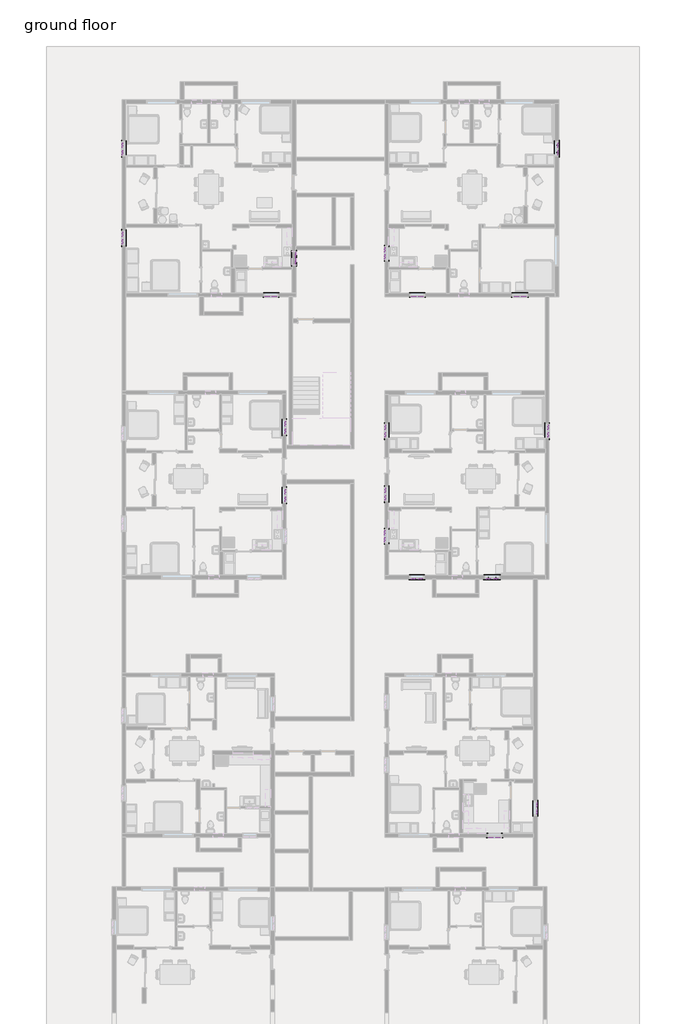
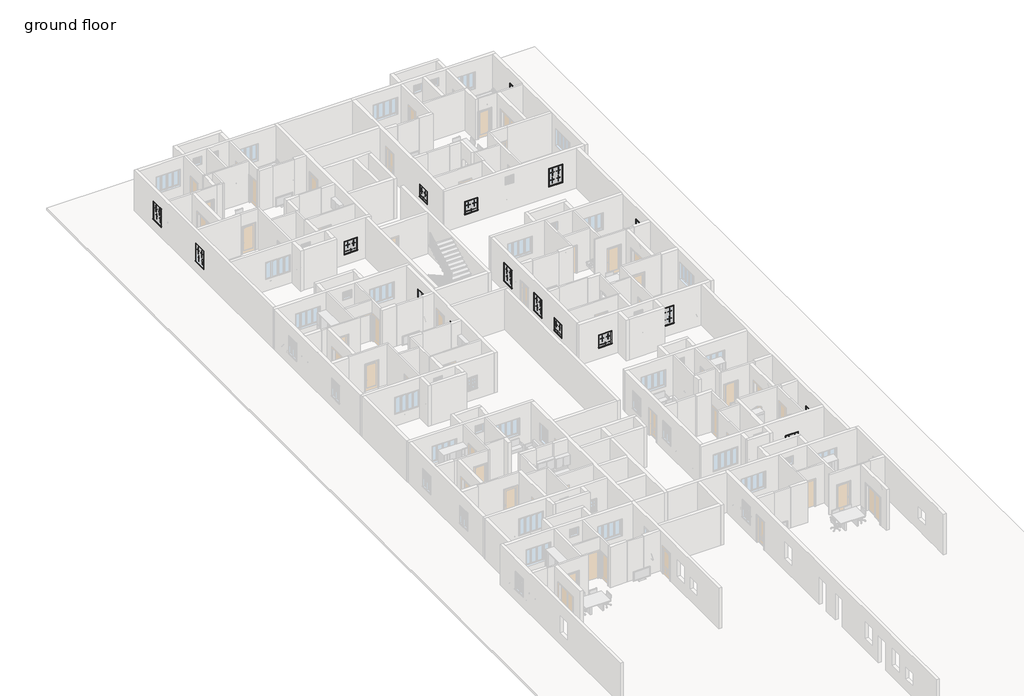
# One storey, part 16 of 16: 100 proxies.
"""IFC4 building model written with IfcOpenShell, lengths in millimetres."""

from ifc_helpers import new_model, si_unit, origin, place, context, project, spatial, transform, mapped, element, save
from components import muntin_pattern_2x2_muntin_pattern_2x2_cd1db81d, muntin_pattern_2x2_muntin_pattern_2x2_7c797e2d, muntin_pattern_2x2_muntin_pattern_2x2_78ce0566, muntin_pattern_2x2_muntin_pattern_2x2_27bf4e5b, muntin_pattern_2x2_muntin_pattern_2x2_8320156c, trim_window_exterior_flat_with_sill_fadbc092, trim_window_exterior_flat_with_sill_41619996, trim_window_interior_flat_picture_frame_db6fc9b7, trim_window_interior_flat_picture_frame_51c85655

model = new_model("IFC4")

# Units and contexts
model_context = context("Model", 3, world=origin())
ifc_project = project(units=[si_unit("LENGTHUNIT", "METRE", prefix="MILLI")], contexts=[model_context])

# Site, building, storey
site = spatial("IfcSite", under=ifc_project)
building = spatial("IfcBuilding", under=site)
storey = spatial("IfcBuildingStorey", under=building, Name="ground floor", Elevation=609.6)

# Proxies
placement = place(None, origin())
muntin_pattern_2x2_muntin_pattern_2x2_shape = muntin_pattern_2x2_muntin_pattern_2x2_cd1db81d(model_context)
element("IfcBuildingElementProxy", 1, Name="Muntin Pattern_2x2 : Muntin Pattern_2x2", ObjectType="Muntin Pattern_2x2 : Muntin Pattern_2x2", at=placement, inside=storey, context=model_context, shape_type="MappedRepresentation", body=[
    mapped(muntin_pattern_2x2_muntin_pattern_2x2_shape, transform((43176.551243, 42287.5965635, 2206.625), x_axis=(0.0, 1.0, 0.0), y_axis=(-1.0, 0.0, 0.0), z_axis=(0.0, 0.0, 1.0))),
])
element("IfcBuildingElementProxy", 2, Name="Muntin Pattern_2x2 : Muntin Pattern_2x2", ObjectType="Muntin Pattern_2x2 : Muntin Pattern_2x2", at=placement, inside=storey, context=model_context, shape_type="MappedRepresentation", body=[
    mapped(muntin_pattern_2x2_muntin_pattern_2x2_shape, transform((43221.001243, 42287.5965635, 1600.2), x_axis=(0.0, 1.0, 0.0), y_axis=(-1.0, 0.0, 0.0), z_axis=(0.0, 0.0, 1.0))),
])
element("IfcBuildingElementProxy", 3, Name="Muntin Pattern_2x2 : Muntin Pattern_2x2", ObjectType="Muntin Pattern_2x2 : Muntin Pattern_2x2", at=placement, inside=storey, context=model_context, shape_type="MappedRepresentation", body=[
    mapped(muntin_pattern_2x2_muntin_pattern_2x2_shape, transform((43176.551243, 47785.5373351, 2206.625), x_axis=(0.0, 1.0, 0.0), y_axis=(-1.0, 0.0, 0.0), z_axis=(0.0, 0.0, 1.0))),
])
element("IfcBuildingElementProxy", 4, Name="Muntin Pattern_2x2 : Muntin Pattern_2x2", ObjectType="Muntin Pattern_2x2 : Muntin Pattern_2x2", at=placement, inside=storey, context=model_context, shape_type="MappedRepresentation", body=[
    mapped(muntin_pattern_2x2_muntin_pattern_2x2_shape, transform((43221.001243, 47785.5373351, 1600.2), x_axis=(0.0, 1.0, 0.0), y_axis=(-1.0, 0.0, 0.0), z_axis=(0.0, 0.0, 1.0))),
])
element("IfcBuildingElementProxy", 5, Name="Muntin Pattern_2x2 : Muntin Pattern_2x2", ObjectType="Muntin Pattern_2x2 : Muntin Pattern_2x2", at=placement, inside=storey, context=model_context, shape_type="MappedRepresentation", body=[
    mapped(muntin_pattern_2x2_muntin_pattern_2x2_shape, transform((67459.9250319, 38468.5059867, 2206.625), x_axis=(-1.0, 0.0, 0.0), y_axis=(0.0, -1.0, 0.0), z_axis=(0.0, 0.0, 1.0))),
])
element("IfcBuildingElementProxy", 6, Name="Muntin Pattern_2x2 : Muntin Pattern_2x2", ObjectType="Muntin Pattern_2x2 : Muntin Pattern_2x2", at=placement, inside=storey, context=model_context, shape_type="MappedRepresentation", body=[
    mapped(muntin_pattern_2x2_muntin_pattern_2x2_shape, transform((67459.9250319, 38512.9559867, 1600.2), x_axis=(-1.0, 0.0, 0.0), y_axis=(0.0, -1.0, 0.0), z_axis=(0.0, 0.0, 1.0))),
])
element("IfcBuildingElementProxy", 7, Name="Muntin Pattern_2x2 : Muntin Pattern_2x2", ObjectType="Muntin Pattern_2x2 : Muntin Pattern_2x2", at=placement, inside=storey, context=model_context, shape_type="MappedRepresentation", body=[
    mapped(muntin_pattern_2x2_muntin_pattern_2x2_shape, transform((70050.1113207, 47329.9248351, 2206.625), x_axis=(0.0, -1.0, 0.0), y_axis=(1.0, 0.0, 0.0), z_axis=(0.0, 0.0, 1.0))),
])
element("IfcBuildingElementProxy", 8, Name="Muntin Pattern_2x2 : Muntin Pattern_2x2", ObjectType="Muntin Pattern_2x2 : Muntin Pattern_2x2", at=placement, inside=storey, context=model_context, shape_type="MappedRepresentation", body=[
    mapped(muntin_pattern_2x2_muntin_pattern_2x2_shape, transform((70005.6613207, 47329.9248351, 1600.2), x_axis=(0.0, -1.0, 0.0), y_axis=(1.0, 0.0, 0.0), z_axis=(0.0, 0.0, 1.0))),
])
element("IfcBuildingElementProxy", 9, Name="Muntin Pattern_2x2 : Muntin Pattern_2x2", ObjectType="Muntin Pattern_2x2 : Muntin Pattern_2x2", at=placement, inside=storey, context=model_context, shape_type="MappedRepresentation", body=[
    mapped(muntin_pattern_2x2_muntin_pattern_2x2_shape, transform((69443.5062819, 29924.6588152, 2206.625), x_axis=(0.0, -1.0, 0.0), y_axis=(1.0, 0.0, 0.0), z_axis=(0.0, 0.0, 1.0))),
])
element("IfcBuildingElementProxy", 10, Name="Muntin Pattern_2x2 : Muntin Pattern_2x2", ObjectType="Muntin Pattern_2x2 : Muntin Pattern_2x2", at=placement, inside=storey, context=model_context, shape_type="MappedRepresentation", body=[
    mapped(muntin_pattern_2x2_muntin_pattern_2x2_shape, transform((69399.0562819, 29924.6588152, 1600.2), x_axis=(0.0, -1.0, 0.0), y_axis=(1.0, 0.0, 0.0), z_axis=(0.0, 0.0, 1.0))),
])
element("IfcBuildingElementProxy", 11, Name="Muntin Pattern_2x2 : Muntin Pattern_2x2", ObjectType="Muntin Pattern_2x2 : Muntin Pattern_2x2", at=placement, inside=storey, context=model_context, shape_type="MappedRepresentation", body=[
    mapped(muntin_pattern_2x2_muntin_pattern_2x2_shape, transform((59391.4562819, 26494.0713152, 2206.625), x_axis=(0.0, 1.0, 0.0), y_axis=(-1.0, 0.0, 0.0), z_axis=(0.0, 0.0, 1.0))),
])
element("IfcBuildingElementProxy", 12, Name="Muntin Pattern_2x2 : Muntin Pattern_2x2", ObjectType="Muntin Pattern_2x2 : Muntin Pattern_2x2", at=placement, inside=storey, context=model_context, shape_type="MappedRepresentation", body=[
    mapped(muntin_pattern_2x2_muntin_pattern_2x2_shape, transform((59435.9062819, 26494.0713152, 1600.2), x_axis=(0.0, 1.0, 0.0), y_axis=(-1.0, 0.0, 0.0), z_axis=(0.0, 0.0, 1.0))),
])
element("IfcBuildingElementProxy", 13, Name="Muntin Pattern_2x2 : Muntin Pattern_2x2", ObjectType="Muntin Pattern_2x2 : Muntin Pattern_2x2", at=placement, inside=storey, context=model_context, shape_type="MappedRepresentation", body=[
    mapped(muntin_pattern_2x2_muntin_pattern_2x2_shape, transform((65744.5920559, 21056.0900652, 2206.625), x_axis=(-1.0, 0.0, 0.0), y_axis=(0.0, -1.0, 0.0), z_axis=(0.0, 0.0, 1.0))),
])
element("IfcBuildingElementProxy", 14, Name="Muntin Pattern_2x2 : Muntin Pattern_2x2", ObjectType="Muntin Pattern_2x2 : Muntin Pattern_2x2", at=placement, inside=storey, context=model_context, shape_type="MappedRepresentation", body=[
    mapped(muntin_pattern_2x2_muntin_pattern_2x2_shape, transform((65744.5920559, 21100.5400652, 1600.2), x_axis=(-1.0, 0.0, 0.0), y_axis=(0.0, -1.0, 0.0), z_axis=(0.0, 0.0, 1.0))),
])
element("IfcBuildingElementProxy", 15, Name="Muntin Pattern_2x2 : Muntin Pattern_2x2", ObjectType="Muntin Pattern_2x2 : Muntin Pattern_2x2", at=placement, inside=storey, context=model_context, shape_type="MappedRepresentation", body=[
    mapped(muntin_pattern_2x2_muntin_pattern_2x2_shape, transform((53228.601243, 25959.8281764, 2206.625), x_axis=(0.0, -1.0, 0.0), y_axis=(1.0, 0.0, 0.0), z_axis=(0.0, 0.0, 1.0))),
])
element("IfcBuildingElementProxy", 16, Name="Muntin Pattern_2x2 : Muntin Pattern_2x2", ObjectType="Muntin Pattern_2x2 : Muntin Pattern_2x2", at=placement, inside=storey, context=model_context, shape_type="MappedRepresentation", body=[
    mapped(muntin_pattern_2x2_muntin_pattern_2x2_shape, transform((53184.151243, 25959.8281764, 1600.2), x_axis=(0.0, -1.0, 0.0), y_axis=(1.0, 0.0, 0.0), z_axis=(0.0, 0.0, 1.0))),
])
element("IfcBuildingElementProxy", 17, Name="Muntin Pattern_2x2 : Muntin Pattern_2x2", ObjectType="Muntin Pattern_2x2 : Muntin Pattern_2x2", at=placement, inside=storey, context=model_context, shape_type="MappedRepresentation", body=[
    mapped(muntin_pattern_2x2_muntin_pattern_2x2_shape, transform((53228.601243, 30153.2588152, 2206.625), x_axis=(0.0, -1.0, 0.0), y_axis=(1.0, 0.0, 0.0), z_axis=(0.0, 0.0, 1.0))),
])
element("IfcBuildingElementProxy", 18, Name="Muntin Pattern_2x2 : Muntin Pattern_2x2", ObjectType="Muntin Pattern_2x2 : Muntin Pattern_2x2", at=placement, inside=storey, context=model_context, shape_type="MappedRepresentation", body=[
    mapped(muntin_pattern_2x2_muntin_pattern_2x2_shape, transform((53184.151243, 30153.2588152, 1600.2), x_axis=(0.0, -1.0, 0.0), y_axis=(1.0, 0.0, 0.0), z_axis=(0.0, 0.0, 1.0))),
])
element("IfcBuildingElementProxy", 19, Name="Muntin Pattern_2x2 : Muntin Pattern_2x2", ObjectType="Muntin Pattern_2x2 : Muntin Pattern_2x2", at=placement, inside=storey, context=model_context, shape_type="MappedRepresentation", body=[
    mapped(muntin_pattern_2x2_muntin_pattern_2x2_shape, transform((59391.4562819, 30380.2713152, 2206.625), x_axis=(0.0, 1.0, 0.0), y_axis=(-1.0, 0.0, 0.0), z_axis=(0.0, 0.0, 1.0))),
])
element("IfcBuildingElementProxy", 20, Name="Muntin Pattern_2x2 : Muntin Pattern_2x2", ObjectType="Muntin Pattern_2x2 : Muntin Pattern_2x2", at=placement, inside=storey, context=model_context, shape_type="MappedRepresentation", body=[
    mapped(muntin_pattern_2x2_muntin_pattern_2x2_shape, transform((59435.9062819, 30380.2713152, 1600.2), x_axis=(0.0, 1.0, 0.0), y_axis=(-1.0, 0.0, 0.0), z_axis=(0.0, 0.0, 1.0))),
])
muntin_pattern_2x2_muntin_pattern_2x2_2_shape = muntin_pattern_2x2_muntin_pattern_2x2_7c797e2d(model_context)
element("IfcBuildingElementProxy", 21, Name="Muntin Pattern_2x2 : Muntin Pattern_2x2", ObjectType="Muntin Pattern_2x2 : Muntin Pattern_2x2", at=placement, inside=storey, context=model_context, shape_type="MappedRepresentation", body=[
    mapped(muntin_pattern_2x2_muntin_pattern_2x2_2_shape, transform((43176.551243, 41831.9840635, 2206.625), x_axis=(0.0, -1.0, 0.0), y_axis=(1.0, 0.0, 0.0), z_axis=(0.0, 0.0, 1.0))),
])
element("IfcBuildingElementProxy", 22, Name="Muntin Pattern_2x2 : Muntin Pattern_2x2", ObjectType="Muntin Pattern_2x2 : Muntin Pattern_2x2", at=placement, inside=storey, context=model_context, shape_type="MappedRepresentation", body=[
    mapped(muntin_pattern_2x2_muntin_pattern_2x2_2_shape, transform((43221.001243, 41831.9840635, 1600.2), x_axis=(0.0, -1.0, 0.0), y_axis=(1.0, 0.0, 0.0), z_axis=(0.0, 0.0, 1.0))),
])
element("IfcBuildingElementProxy", 23, Name="Muntin Pattern_2x2 : Muntin Pattern_2x2", ObjectType="Muntin Pattern_2x2 : Muntin Pattern_2x2", at=placement, inside=storey, context=model_context, shape_type="MappedRepresentation", body=[
    mapped(muntin_pattern_2x2_muntin_pattern_2x2_2_shape, transform((43176.551243, 47329.9248351, 2206.625), x_axis=(0.0, -1.0, 0.0), y_axis=(1.0, 0.0, 0.0), z_axis=(0.0, 0.0, 1.0))),
])
element("IfcBuildingElementProxy", 24, Name="Muntin Pattern_2x2 : Muntin Pattern_2x2", ObjectType="Muntin Pattern_2x2 : Muntin Pattern_2x2", at=placement, inside=storey, context=model_context, shape_type="MappedRepresentation", body=[
    mapped(muntin_pattern_2x2_muntin_pattern_2x2_2_shape, transform((43221.001243, 47329.9248351, 1600.2), x_axis=(0.0, -1.0, 0.0), y_axis=(1.0, 0.0, 0.0), z_axis=(0.0, 0.0, 1.0))),
])
element("IfcBuildingElementProxy", 25, Name="Muntin Pattern_2x2 : Muntin Pattern_2x2", ObjectType="Muntin Pattern_2x2 : Muntin Pattern_2x2", at=placement, inside=storey, context=model_context, shape_type="MappedRepresentation", body=[
    mapped(muntin_pattern_2x2_muntin_pattern_2x2_2_shape, transform((67915.5375319, 38468.5059867, 2206.625), x_axis=(1.0, 0.0, 0.0), y_axis=(0.0, 1.0, 0.0), z_axis=(0.0, 0.0, 1.0))),
])
element("IfcBuildingElementProxy", 26, Name="Muntin Pattern_2x2 : Muntin Pattern_2x2", ObjectType="Muntin Pattern_2x2 : Muntin Pattern_2x2", at=placement, inside=storey, context=model_context, shape_type="MappedRepresentation", body=[
    mapped(muntin_pattern_2x2_muntin_pattern_2x2_2_shape, transform((67915.5375319, 38512.9559867, 1600.2), x_axis=(1.0, 0.0, 0.0), y_axis=(0.0, 1.0, 0.0), z_axis=(0.0, 0.0, 1.0))),
])
element("IfcBuildingElementProxy", 27, Name="Muntin Pattern_2x2 : Muntin Pattern_2x2", ObjectType="Muntin Pattern_2x2 : Muntin Pattern_2x2", at=placement, inside=storey, context=model_context, shape_type="MappedRepresentation", body=[
    mapped(muntin_pattern_2x2_muntin_pattern_2x2_2_shape, transform((70050.1113207, 47785.5373351, 2206.625), x_axis=(0.0, 1.0, 0.0), y_axis=(-1.0, 0.0, 0.0), z_axis=(0.0, 0.0, 1.0))),
])
element("IfcBuildingElementProxy", 28, Name="Muntin Pattern_2x2 : Muntin Pattern_2x2", ObjectType="Muntin Pattern_2x2 : Muntin Pattern_2x2", at=placement, inside=storey, context=model_context, shape_type="MappedRepresentation", body=[
    mapped(muntin_pattern_2x2_muntin_pattern_2x2_2_shape, transform((70005.6613207, 47785.5373351, 1600.2), x_axis=(0.0, 1.0, 0.0), y_axis=(-1.0, 0.0, 0.0), z_axis=(0.0, 0.0, 1.0))),
])
element("IfcBuildingElementProxy", 29, Name="Muntin Pattern_2x2 : Muntin Pattern_2x2", ObjectType="Muntin Pattern_2x2 : Muntin Pattern_2x2", at=placement, inside=storey, context=model_context, shape_type="MappedRepresentation", body=[
    mapped(muntin_pattern_2x2_muntin_pattern_2x2_2_shape, transform((69443.5062819, 30380.2713152, 2206.625), x_axis=(0.0, 1.0, 0.0), y_axis=(-1.0, 0.0, 0.0), z_axis=(0.0, 0.0, 1.0))),
])
element("IfcBuildingElementProxy", 30, Name="Muntin Pattern_2x2 : Muntin Pattern_2x2", ObjectType="Muntin Pattern_2x2 : Muntin Pattern_2x2", at=placement, inside=storey, context=model_context, shape_type="MappedRepresentation", body=[
    mapped(muntin_pattern_2x2_muntin_pattern_2x2_2_shape, transform((69399.0562819, 30380.2713152, 1600.2), x_axis=(0.0, 1.0, 0.0), y_axis=(-1.0, 0.0, 0.0), z_axis=(0.0, 0.0, 1.0))),
])
element("IfcBuildingElementProxy", 31, Name="Muntin Pattern_2x2 : Muntin Pattern_2x2", ObjectType="Muntin Pattern_2x2 : Muntin Pattern_2x2", at=placement, inside=storey, context=model_context, shape_type="MappedRepresentation", body=[
    mapped(muntin_pattern_2x2_muntin_pattern_2x2_2_shape, transform((59391.4562819, 26038.4588152, 2206.625), x_axis=(0.0, -1.0, 0.0), y_axis=(1.0, 0.0, 0.0), z_axis=(0.0, 0.0, 1.0))),
])
element("IfcBuildingElementProxy", 32, Name="Muntin Pattern_2x2 : Muntin Pattern_2x2", ObjectType="Muntin Pattern_2x2 : Muntin Pattern_2x2", at=placement, inside=storey, context=model_context, shape_type="MappedRepresentation", body=[
    mapped(muntin_pattern_2x2_muntin_pattern_2x2_2_shape, transform((59435.9062819, 26038.4588152, 1600.2), x_axis=(0.0, -1.0, 0.0), y_axis=(1.0, 0.0, 0.0), z_axis=(0.0, 0.0, 1.0))),
])
element("IfcBuildingElementProxy", 33, Name="Muntin Pattern_2x2 : Muntin Pattern_2x2", ObjectType="Muntin Pattern_2x2 : Muntin Pattern_2x2", at=placement, inside=storey, context=model_context, shape_type="MappedRepresentation", body=[
    mapped(muntin_pattern_2x2_muntin_pattern_2x2_2_shape, transform((66200.2045559, 21056.0900652, 2206.625), x_axis=(1.0, 0.0, 0.0), y_axis=(0.0, 1.0, 0.0), z_axis=(0.0, 0.0, 1.0))),
])
element("IfcBuildingElementProxy", 34, Name="Muntin Pattern_2x2 : Muntin Pattern_2x2", ObjectType="Muntin Pattern_2x2 : Muntin Pattern_2x2", at=placement, inside=storey, context=model_context, shape_type="MappedRepresentation", body=[
    mapped(muntin_pattern_2x2_muntin_pattern_2x2_2_shape, transform((66200.2045559, 21100.5400652, 1600.2), x_axis=(1.0, 0.0, 0.0), y_axis=(0.0, 1.0, 0.0), z_axis=(0.0, 0.0, 1.0))),
])
element("IfcBuildingElementProxy", 35, Name="Muntin Pattern_2x2 : Muntin Pattern_2x2", ObjectType="Muntin Pattern_2x2 : Muntin Pattern_2x2", at=placement, inside=storey, context=model_context, shape_type="MappedRepresentation", body=[
    mapped(muntin_pattern_2x2_muntin_pattern_2x2_2_shape, transform((53228.601243, 26415.4406764, 2206.625), x_axis=(0.0, 1.0, 0.0), y_axis=(-1.0, 0.0, 0.0), z_axis=(0.0, 0.0, 1.0))),
])
element("IfcBuildingElementProxy", 36, Name="Muntin Pattern_2x2 : Muntin Pattern_2x2", ObjectType="Muntin Pattern_2x2 : Muntin Pattern_2x2", at=placement, inside=storey, context=model_context, shape_type="MappedRepresentation", body=[
    mapped(muntin_pattern_2x2_muntin_pattern_2x2_2_shape, transform((53184.151243, 26415.4406764, 1600.2), x_axis=(0.0, 1.0, 0.0), y_axis=(-1.0, 0.0, 0.0), z_axis=(0.0, 0.0, 1.0))),
])
element("IfcBuildingElementProxy", 37, Name="Muntin Pattern_2x2 : Muntin Pattern_2x2", ObjectType="Muntin Pattern_2x2 : Muntin Pattern_2x2", at=placement, inside=storey, context=model_context, shape_type="MappedRepresentation", body=[
    mapped(muntin_pattern_2x2_muntin_pattern_2x2_2_shape, transform((53228.601243, 30608.8713152, 2206.625), x_axis=(0.0, 1.0, 0.0), y_axis=(-1.0, 0.0, 0.0), z_axis=(0.0, 0.0, 1.0))),
])
element("IfcBuildingElementProxy", 38, Name="Muntin Pattern_2x2 : Muntin Pattern_2x2", ObjectType="Muntin Pattern_2x2 : Muntin Pattern_2x2", at=placement, inside=storey, context=model_context, shape_type="MappedRepresentation", body=[
    mapped(muntin_pattern_2x2_muntin_pattern_2x2_2_shape, transform((53184.151243, 30608.8713152, 1600.2), x_axis=(0.0, 1.0, 0.0), y_axis=(-1.0, 0.0, 0.0), z_axis=(0.0, 0.0, 1.0))),
])
element("IfcBuildingElementProxy", 39, Name="Muntin Pattern_2x2 : Muntin Pattern_2x2", ObjectType="Muntin Pattern_2x2 : Muntin Pattern_2x2", at=placement, inside=storey, context=model_context, shape_type="MappedRepresentation", body=[
    mapped(muntin_pattern_2x2_muntin_pattern_2x2_2_shape, transform((59391.4562819, 29924.6588152, 2206.625), x_axis=(0.0, -1.0, 0.0), y_axis=(1.0, 0.0, 0.0), z_axis=(0.0, 0.0, 1.0))),
])
element("IfcBuildingElementProxy", 40, Name="Muntin Pattern_2x2 : Muntin Pattern_2x2", ObjectType="Muntin Pattern_2x2 : Muntin Pattern_2x2", at=placement, inside=storey, context=model_context, shape_type="MappedRepresentation", body=[
    mapped(muntin_pattern_2x2_muntin_pattern_2x2_2_shape, transform((59435.9062819, 29924.6588152, 1600.2), x_axis=(0.0, -1.0, 0.0), y_axis=(1.0, 0.0, 0.0), z_axis=(0.0, 0.0, 1.0))),
])
muntin_pattern_2x2_muntin_pattern_2x2_3_shape = muntin_pattern_2x2_muntin_pattern_2x2_78ce0566(model_context)
element("IfcBuildingElementProxy", 41, Name="Muntin Pattern_2x2 : Muntin Pattern_2x2", ObjectType="Muntin Pattern_2x2 : Muntin Pattern_2x2", at=placement, inside=storey, context=model_context, shape_type="MappedRepresentation", body=[
    mapped(muntin_pattern_2x2_muntin_pattern_2x2_3_shape, transform((53860.6062819, 41023.3668028, 2203.45), x_axis=(0.0, -1.0, 0.0), y_axis=(1.0, 0.0, 0.0), z_axis=(0.0, 0.0, 1.0))),
])
element("IfcBuildingElementProxy", 42, Name="Muntin Pattern_2x2 : Muntin Pattern_2x2", ObjectType="Muntin Pattern_2x2 : Muntin Pattern_2x2", at=placement, inside=storey, context=model_context, shape_type="MappedRepresentation", body=[
    mapped(muntin_pattern_2x2_muntin_pattern_2x2_3_shape, transform((52547.7437819, 38443.1059867, 1898.65), x_axis=(-1.0, 0.0, 0.0), y_axis=(0.0, -1.0, 0.0), z_axis=(0.0, 0.0, 1.0))),
])
element("IfcBuildingElementProxy", 43, Name="Muntin Pattern_2x2 : Muntin Pattern_2x2", ObjectType="Muntin Pattern_2x2 : Muntin Pattern_2x2", at=placement, inside=storey, context=model_context, shape_type="MappedRepresentation", body=[
    mapped(muntin_pattern_2x2_muntin_pattern_2x2_3_shape, transform((59366.0562819, 40899.5418028, 1898.65), x_axis=(0.0, 1.0, 0.0), y_axis=(-1.0, 0.0, 0.0), z_axis=(0.0, 0.0, 1.0))),
])
element("IfcBuildingElementProxy", 44, Name="Muntin Pattern_2x2 : Muntin Pattern_2x2", ObjectType="Muntin Pattern_2x2 : Muntin Pattern_2x2", at=placement, inside=storey, context=model_context, shape_type="MappedRepresentation", body=[
    mapped(muntin_pattern_2x2_muntin_pattern_2x2_3_shape, transform((61574.7147227, 38443.1059867, 1898.65), x_axis=(-1.0, 0.0, 0.0), y_axis=(0.0, -1.0, 0.0), z_axis=(0.0, 0.0, 1.0))),
])
element("IfcBuildingElementProxy", 45, Name="Muntin Pattern_2x2 : Muntin Pattern_2x2", ObjectType="Muntin Pattern_2x2 : Muntin Pattern_2x2", at=placement, inside=storey, context=model_context, shape_type="MappedRepresentation", body=[
    mapped(muntin_pattern_2x2_muntin_pattern_2x2_3_shape, transform((59366.0562819, 23454.8025652, 1898.65), x_axis=(0.0, 1.0, 0.0), y_axis=(-1.0, 0.0, 0.0), z_axis=(0.0, 0.0, 1.0))),
])
element("IfcBuildingElementProxy", 46, Name="Muntin Pattern_2x2 : Muntin Pattern_2x2", ObjectType="Muntin Pattern_2x2 : Muntin Pattern_2x2", at=placement, inside=storey, context=model_context, shape_type="MappedRepresentation", body=[
    mapped(muntin_pattern_2x2_muntin_pattern_2x2_3_shape, transform((61552.0437819, 21030.6900652, 1898.65), x_axis=(-1.0, 0.0, 0.0), y_axis=(0.0, -1.0, 0.0), z_axis=(0.0, 0.0, 1.0))),
])
element("IfcBuildingElementProxy", 47, Name="Muntin Pattern_2x2 : Muntin Pattern_2x2", ObjectType="Muntin Pattern_2x2 : Muntin Pattern_2x2", at=placement, inside=storey, context=model_context, shape_type="MappedRepresentation", body=[
    mapped(muntin_pattern_2x2_muntin_pattern_2x2_3_shape, transform((68745.0062819, 7100.3775652, 1898.65), x_axis=(0.0, -1.0, 0.0), y_axis=(1.0, 0.0, 0.0), z_axis=(0.0, 0.0, 1.0))),
])
element("IfcBuildingElementProxy", 48, Name="Muntin Pattern_2x2 : Muntin Pattern_2x2", ObjectType="Muntin Pattern_2x2 : Muntin Pattern_2x2", at=placement, inside=storey, context=model_context, shape_type="MappedRepresentation", body=[
    mapped(muntin_pattern_2x2_muntin_pattern_2x2_3_shape, transform((66346.2937819, 5104.8900652, 1898.65), x_axis=(-1.0, 0.0, 0.0), y_axis=(0.0, -1.0, 0.0), z_axis=(0.0, 0.0, 1.0))),
])
muntin_pattern_2x2_muntin_pattern_2x2_4_shape = muntin_pattern_2x2_muntin_pattern_2x2_27bf4e5b(model_context)
element("IfcBuildingElementProxy", 49, Name="Muntin Pattern_2x2 : Muntin Pattern_2x2", ObjectType="Muntin Pattern_2x2 : Muntin Pattern_2x2", at=placement, inside=storey, context=model_context, shape_type="MappedRepresentation", body=[
    mapped(muntin_pattern_2x2_muntin_pattern_2x2_4_shape, transform((53860.6062819, 40594.7418028, 2203.45), x_axis=(0.0, 1.0, 0.0), y_axis=(-1.0, 0.0, 0.0), z_axis=(0.0, 0.0, 1.0))),
])
element("IfcBuildingElementProxy", 50, Name="Muntin Pattern_2x2 : Muntin Pattern_2x2", ObjectType="Muntin Pattern_2x2 : Muntin Pattern_2x2", at=placement, inside=storey, context=model_context, shape_type="MappedRepresentation", body=[
    mapped(muntin_pattern_2x2_muntin_pattern_2x2_4_shape, transform((52119.1187819, 38443.1059867, 1898.65), x_axis=(1.0, 0.0, 0.0), y_axis=(0.0, 1.0, 0.0), z_axis=(0.0, 0.0, 1.0))),
])
element("IfcBuildingElementProxy", 51, Name="Muntin Pattern_2x2 : Muntin Pattern_2x2", ObjectType="Muntin Pattern_2x2 : Muntin Pattern_2x2", at=placement, inside=storey, context=model_context, shape_type="MappedRepresentation", body=[
    mapped(muntin_pattern_2x2_muntin_pattern_2x2_4_shape, transform((59366.0562819, 41328.1668028, 1898.65), x_axis=(0.0, -1.0, 0.0), y_axis=(1.0, 0.0, 0.0), z_axis=(0.0, 0.0, 1.0))),
])
element("IfcBuildingElementProxy", 52, Name="Muntin Pattern_2x2 : Muntin Pattern_2x2", ObjectType="Muntin Pattern_2x2 : Muntin Pattern_2x2", at=placement, inside=storey, context=model_context, shape_type="MappedRepresentation", body=[
    mapped(muntin_pattern_2x2_muntin_pattern_2x2_4_shape, transform((61146.0897227, 38443.1059867, 1898.65), x_axis=(1.0, 0.0, 0.0), y_axis=(0.0, 1.0, 0.0), z_axis=(0.0, 0.0, 1.0))),
])
element("IfcBuildingElementProxy", 53, Name="Muntin Pattern_2x2 : Muntin Pattern_2x2", ObjectType="Muntin Pattern_2x2 : Muntin Pattern_2x2", at=placement, inside=storey, context=model_context, shape_type="MappedRepresentation", body=[
    mapped(muntin_pattern_2x2_muntin_pattern_2x2_4_shape, transform((59366.0562819, 23883.4275652, 1898.65), x_axis=(0.0, -1.0, 0.0), y_axis=(1.0, 0.0, 0.0), z_axis=(0.0, 0.0, 1.0))),
])
element("IfcBuildingElementProxy", 54, Name="Muntin Pattern_2x2 : Muntin Pattern_2x2", ObjectType="Muntin Pattern_2x2 : Muntin Pattern_2x2", at=placement, inside=storey, context=model_context, shape_type="MappedRepresentation", body=[
    mapped(muntin_pattern_2x2_muntin_pattern_2x2_4_shape, transform((61123.4187819, 21030.6900652, 1898.65), x_axis=(1.0, 0.0, 0.0), y_axis=(0.0, 1.0, 0.0), z_axis=(0.0, 0.0, 1.0))),
])
element("IfcBuildingElementProxy", 55, Name="Muntin Pattern_2x2 : Muntin Pattern_2x2", ObjectType="Muntin Pattern_2x2 : Muntin Pattern_2x2", at=placement, inside=storey, context=model_context, shape_type="MappedRepresentation", body=[
    mapped(muntin_pattern_2x2_muntin_pattern_2x2_4_shape, transform((68745.0062819, 6671.7525652, 1898.65), x_axis=(0.0, 1.0, 0.0), y_axis=(-1.0, 0.0, 0.0), z_axis=(0.0, 0.0, 1.0))),
])
element("IfcBuildingElementProxy", 56, Name="Muntin Pattern_2x2 : Muntin Pattern_2x2", ObjectType="Muntin Pattern_2x2 : Muntin Pattern_2x2", at=placement, inside=storey, context=model_context, shape_type="MappedRepresentation", body=[
    mapped(muntin_pattern_2x2_muntin_pattern_2x2_4_shape, transform((65917.6687819, 5104.8900652, 1898.65), x_axis=(1.0, 0.0, 0.0), y_axis=(0.0, 1.0, 0.0), z_axis=(0.0, 0.0, 1.0))),
])
muntin_pattern_2x2_muntin_pattern_2x2_5_shape = muntin_pattern_2x2_muntin_pattern_2x2_8320156c(model_context)
element("IfcBuildingElementProxy", 57, Name="Muntin Pattern_2x2 : Muntin Pattern_2x2", ObjectType="Muntin Pattern_2x2 : Muntin Pattern_2x2", at=placement, inside=storey, context=model_context, shape_type="MappedRepresentation", body=[
    mapped(muntin_pattern_2x2_muntin_pattern_2x2_5_shape, transform((53860.6062819, 40809.0543028, 1898.65), x_axis=(0.0, 1.0, 0.0), y_axis=(-1.0, 0.0, 0.0), z_axis=(0.0, 0.0, 1.0))),
])
element("IfcBuildingElementProxy", 58, Name="Muntin Pattern_2x2 : Muntin Pattern_2x2", ObjectType="Muntin Pattern_2x2 : Muntin Pattern_2x2", at=placement, inside=storey, context=model_context, shape_type="MappedRepresentation", body=[
    mapped(muntin_pattern_2x2_muntin_pattern_2x2_5_shape, transform((52333.4312819, 38443.1059867, 1593.85), x_axis=(1.0, 0.0, 0.0), y_axis=(0.0, 1.0, 0.0), z_axis=(0.0, 0.0, 1.0))),
])
element("IfcBuildingElementProxy", 59, Name="Muntin Pattern_2x2 : Muntin Pattern_2x2", ObjectType="Muntin Pattern_2x2 : Muntin Pattern_2x2", at=placement, inside=storey, context=model_context, shape_type="MappedRepresentation", body=[
    mapped(muntin_pattern_2x2_muntin_pattern_2x2_5_shape, transform((59366.0562819, 41113.8543028, 1593.85), x_axis=(0.0, -1.0, 0.0), y_axis=(1.0, 0.0, 0.0), z_axis=(0.0, 0.0, 1.0))),
])
element("IfcBuildingElementProxy", 60, Name="Muntin Pattern_2x2 : Muntin Pattern_2x2", ObjectType="Muntin Pattern_2x2 : Muntin Pattern_2x2", at=placement, inside=storey, context=model_context, shape_type="MappedRepresentation", body=[
    mapped(muntin_pattern_2x2_muntin_pattern_2x2_5_shape, transform((61360.4022227, 38443.1059867, 1593.85), x_axis=(1.0, 0.0, 0.0), y_axis=(0.0, 1.0, 0.0), z_axis=(0.0, 0.0, 1.0))),
])
element("IfcBuildingElementProxy", 61, Name="Muntin Pattern_2x2 : Muntin Pattern_2x2", ObjectType="Muntin Pattern_2x2 : Muntin Pattern_2x2", at=placement, inside=storey, context=model_context, shape_type="MappedRepresentation", body=[
    mapped(muntin_pattern_2x2_muntin_pattern_2x2_5_shape, transform((59366.0562819, 23669.1150652, 1593.85), x_axis=(0.0, -1.0, 0.0), y_axis=(1.0, 0.0, 0.0), z_axis=(0.0, 0.0, 1.0))),
])
element("IfcBuildingElementProxy", 62, Name="Muntin Pattern_2x2 : Muntin Pattern_2x2", ObjectType="Muntin Pattern_2x2 : Muntin Pattern_2x2", at=placement, inside=storey, context=model_context, shape_type="MappedRepresentation", body=[
    mapped(muntin_pattern_2x2_muntin_pattern_2x2_5_shape, transform((61337.7312819, 21030.6900652, 1593.85), x_axis=(1.0, 0.0, 0.0), y_axis=(0.0, 1.0, 0.0), z_axis=(0.0, 0.0, 1.0))),
])
element("IfcBuildingElementProxy", 63, Name="Muntin Pattern_2x2 : Muntin Pattern_2x2", ObjectType="Muntin Pattern_2x2 : Muntin Pattern_2x2", at=placement, inside=storey, context=model_context, shape_type="MappedRepresentation", body=[
    mapped(muntin_pattern_2x2_muntin_pattern_2x2_5_shape, transform((68745.0062819, 6886.0650652, 1593.85), x_axis=(0.0, 1.0, 0.0), y_axis=(-1.0, 0.0, 0.0), z_axis=(0.0, 0.0, 1.0))),
])
element("IfcBuildingElementProxy", 64, Name="Muntin Pattern_2x2 : Muntin Pattern_2x2", ObjectType="Muntin Pattern_2x2 : Muntin Pattern_2x2", at=placement, inside=storey, context=model_context, shape_type="MappedRepresentation", body=[
    mapped(muntin_pattern_2x2_muntin_pattern_2x2_5_shape, transform((66131.9812819, 5104.8900652, 1593.85), x_axis=(1.0, 0.0, 0.0), y_axis=(0.0, 1.0, 0.0), z_axis=(0.0, 0.0, 1.0))),
])
trim_window_exterior_flat_with_sill_shape = trim_window_exterior_flat_with_sill_fadbc092(model_context)
element("IfcBuildingElementProxy", 65, Name="Trim-Window-Exterior-Flat : with Sill", ObjectType="Trim-Window-Exterior-Flat : with Sill", at=placement, inside=storey, context=model_context, shape_type="MappedRepresentation", body=[
    mapped(trim_window_exterior_flat_with_sill_shape, transform((43141.626243, 42059.7903135, 2844.8), x_axis=(0.0, -1.0, 0.0), y_axis=(0.0, 0.0, 1.0), z_axis=(-1.0, 0.0, 0.0))),
])
element("IfcBuildingElementProxy", 66, Name="Trim-Window-Exterior-Flat : with Sill", ObjectType="Trim-Window-Exterior-Flat : with Sill", at=placement, inside=storey, context=model_context, shape_type="MappedRepresentation", body=[
    mapped(trim_window_exterior_flat_with_sill_shape, transform((43141.626243, 47557.7310851, 2844.8), x_axis=(0.0, -1.0, 0.0), y_axis=(0.0, 0.0, 1.0), z_axis=(-1.0, 0.0, 0.0))),
])
element("IfcBuildingElementProxy", 67, Name="Trim-Window-Exterior-Flat : with Sill", ObjectType="Trim-Window-Exterior-Flat : with Sill", at=placement, inside=storey, context=model_context, shape_type="MappedRepresentation", body=[
    mapped(trim_window_exterior_flat_with_sill_shape, transform((67687.7312819, 38433.5809867, 2844.8), x_axis=(1.0, 0.0, 0.0), y_axis=(0.0, 0.0, 1.0), z_axis=(0.0, -1.0, 0.0))),
])
element("IfcBuildingElementProxy", 68, Name="Trim-Window-Exterior-Flat : with Sill", ObjectType="Trim-Window-Exterior-Flat : with Sill", at=placement, inside=storey, context=model_context, shape_type="MappedRepresentation", body=[
    mapped(trim_window_exterior_flat_with_sill_shape, transform((70085.0363207, 47557.7310851, 2844.8), x_axis=(0.0, 1.0, 0.0), y_axis=(0.0, 0.0, 1.0), z_axis=(1.0, 0.0, 0.0))),
])
element("IfcBuildingElementProxy", 69, Name="Trim-Window-Exterior-Flat : with Sill", ObjectType="Trim-Window-Exterior-Flat : with Sill", at=placement, inside=storey, context=model_context, shape_type="MappedRepresentation", body=[
    mapped(trim_window_exterior_flat_with_sill_shape, transform((69478.4312819, 30152.4650652, 2844.8), x_axis=(0.0, 1.0, 0.0), y_axis=(0.0, 0.0, 1.0), z_axis=(1.0, 0.0, 0.0))),
])
element("IfcBuildingElementProxy", 70, Name="Trim-Window-Exterior-Flat : with Sill", ObjectType="Trim-Window-Exterior-Flat : with Sill", at=placement, inside=storey, context=model_context, shape_type="MappedRepresentation", body=[
    mapped(trim_window_exterior_flat_with_sill_shape, transform((59356.5312819, 26266.2650652, 2844.8), x_axis=(0.0, -1.0, 0.0), y_axis=(0.0, 0.0, 1.0), z_axis=(-1.0, 0.0, 0.0))),
])
element("IfcBuildingElementProxy", 71, Name="Trim-Window-Exterior-Flat : with Sill", ObjectType="Trim-Window-Exterior-Flat : with Sill", at=placement, inside=storey, context=model_context, shape_type="MappedRepresentation", body=[
    mapped(trim_window_exterior_flat_with_sill_shape, transform((65972.3983059, 21021.1650652, 2844.8), x_axis=(1.0, 0.0, 0.0), y_axis=(0.0, 0.0, 1.0), z_axis=(0.0, -1.0, 0.0))),
])
element("IfcBuildingElementProxy", 72, Name="Trim-Window-Exterior-Flat : with Sill", ObjectType="Trim-Window-Exterior-Flat : with Sill", at=placement, inside=storey, context=model_context, shape_type="MappedRepresentation", body=[
    mapped(trim_window_exterior_flat_with_sill_shape, transform((53263.526243, 26187.6344264, 2844.8), x_axis=(0.0, 1.0, 0.0), y_axis=(0.0, 0.0, 1.0), z_axis=(1.0, 0.0, 0.0))),
])
element("IfcBuildingElementProxy", 73, Name="Trim-Window-Exterior-Flat : with Sill", ObjectType="Trim-Window-Exterior-Flat : with Sill", at=placement, inside=storey, context=model_context, shape_type="MappedRepresentation", body=[
    mapped(trim_window_exterior_flat_with_sill_shape, transform((53263.526243, 30381.0650652, 2844.8), x_axis=(0.0, 1.0, 0.0), y_axis=(0.0, 0.0, 1.0), z_axis=(1.0, 0.0, 0.0))),
])
element("IfcBuildingElementProxy", 74, Name="Trim-Window-Exterior-Flat : with Sill", ObjectType="Trim-Window-Exterior-Flat : with Sill", at=placement, inside=storey, context=model_context, shape_type="MappedRepresentation", body=[
    mapped(trim_window_exterior_flat_with_sill_shape, transform((59356.5312819, 30152.4650652, 2844.8), x_axis=(0.0, -1.0, 0.0), y_axis=(0.0, 0.0, 1.0), z_axis=(-1.0, 0.0, 0.0))),
])
trim_window_exterior_flat_with_sill_2_shape = trim_window_exterior_flat_with_sill_41619996(model_context)
element("IfcBuildingElementProxy", 75, Name="Trim-Window-Exterior-Flat : with Sill", ObjectType="Trim-Window-Exterior-Flat : with Sill", at=placement, inside=storey, context=model_context, shape_type="MappedRepresentation", body=[
    mapped(trim_window_exterior_flat_with_sill_2_shape, transform((53870.1312819, 40809.0543028, 2743.2), x_axis=(0.0, 1.0, 0.0), y_axis=(0.0, 0.0, 1.0), z_axis=(1.0, 0.0, 0.0))),
])
element("IfcBuildingElementProxy", 76, Name="Trim-Window-Exterior-Flat : with Sill", ObjectType="Trim-Window-Exterior-Flat : with Sill", at=placement, inside=storey, context=model_context, shape_type="MappedRepresentation", body=[
    mapped(trim_window_exterior_flat_with_sill_2_shape, transform((52333.4312819, 38433.5809867, 2438.4), x_axis=(1.0, 0.0, 0.0), y_axis=(0.0, 0.0, 1.0), z_axis=(0.0, -1.0, 0.0))),
])
element("IfcBuildingElementProxy", 77, Name="Trim-Window-Exterior-Flat : with Sill", ObjectType="Trim-Window-Exterior-Flat : with Sill", at=placement, inside=storey, context=model_context, shape_type="MappedRepresentation", body=[
    mapped(trim_window_exterior_flat_with_sill_2_shape, transform((59356.5312819, 41113.8543028, 2438.4), x_axis=(0.0, -1.0, 0.0), y_axis=(0.0, 0.0, 1.0), z_axis=(-1.0, 0.0, 0.0))),
])
element("IfcBuildingElementProxy", 78, Name="Trim-Window-Exterior-Flat : with Sill", ObjectType="Trim-Window-Exterior-Flat : with Sill", at=placement, inside=storey, context=model_context, shape_type="MappedRepresentation", body=[
    mapped(trim_window_exterior_flat_with_sill_2_shape, transform((61360.4022227, 38433.5809867, 2438.4), x_axis=(1.0, 0.0, 0.0), y_axis=(0.0, 0.0, 1.0), z_axis=(0.0, -1.0, 0.0))),
])
element("IfcBuildingElementProxy", 79, Name="Trim-Window-Exterior-Flat : with Sill", ObjectType="Trim-Window-Exterior-Flat : with Sill", at=placement, inside=storey, context=model_context, shape_type="MappedRepresentation", body=[
    mapped(trim_window_exterior_flat_with_sill_2_shape, transform((59356.5312819, 23669.1150652, 2438.4), x_axis=(0.0, -1.0, 0.0), y_axis=(0.0, 0.0, 1.0), z_axis=(-1.0, 0.0, 0.0))),
])
element("IfcBuildingElementProxy", 80, Name="Trim-Window-Exterior-Flat : with Sill", ObjectType="Trim-Window-Exterior-Flat : with Sill", at=placement, inside=storey, context=model_context, shape_type="MappedRepresentation", body=[
    mapped(trim_window_exterior_flat_with_sill_2_shape, transform((61337.7312819, 21021.1650652, 2438.4), x_axis=(1.0, 0.0, 0.0), y_axis=(0.0, 0.0, 1.0), z_axis=(0.0, -1.0, 0.0))),
])
element("IfcBuildingElementProxy", 81, Name="Trim-Window-Exterior-Flat : with Sill", ObjectType="Trim-Window-Exterior-Flat : with Sill", at=placement, inside=storey, context=model_context, shape_type="MappedRepresentation", body=[
    mapped(trim_window_exterior_flat_with_sill_2_shape, transform((68754.5312819, 6886.0650652, 2438.4), x_axis=(0.0, 1.0, 0.0), y_axis=(0.0, 0.0, 1.0), z_axis=(1.0, 0.0, 0.0))),
])
element("IfcBuildingElementProxy", 82, Name="Trim-Window-Exterior-Flat : with Sill", ObjectType="Trim-Window-Exterior-Flat : with Sill", at=placement, inside=storey, context=model_context, shape_type="MappedRepresentation", body=[
    mapped(trim_window_exterior_flat_with_sill_2_shape, transform((66131.9812819, 5095.3650652, 2438.4), x_axis=(1.0, 0.0, 0.0), y_axis=(0.0, 0.0, 1.0), z_axis=(0.0, -1.0, 0.0))),
])
trim_window_interior_flat_picture_frame_shape = trim_window_interior_flat_picture_frame_db6fc9b7(model_context)
element("IfcBuildingElementProxy", 83, Name="Trim-Window-Interior-Flat : Picture Frame", ObjectType="Trim-Window-Interior-Flat : Picture Frame", at=placement, inside=storey, context=model_context, shape_type="MappedRepresentation", body=[
    mapped(trim_window_interior_flat_picture_frame_shape, transform((43370.226243, 42059.7903135, 2844.8), x_axis=(0.0, 1.0, 0.0), y_axis=(0.0, 0.0, 1.0), z_axis=(1.0, 0.0, 0.0))),
])
element("IfcBuildingElementProxy", 84, Name="Trim-Window-Interior-Flat : Picture Frame", ObjectType="Trim-Window-Interior-Flat : Picture Frame", at=placement, inside=storey, context=model_context, shape_type="MappedRepresentation", body=[
    mapped(trim_window_interior_flat_picture_frame_shape, transform((43370.226243, 47557.7310851, 2844.8), x_axis=(0.0, 1.0, 0.0), y_axis=(0.0, 0.0, 1.0), z_axis=(1.0, 0.0, 0.0))),
])
element("IfcBuildingElementProxy", 85, Name="Trim-Window-Interior-Flat : Picture Frame", ObjectType="Trim-Window-Interior-Flat : Picture Frame", at=placement, inside=storey, context=model_context, shape_type="MappedRepresentation", body=[
    mapped(trim_window_interior_flat_picture_frame_shape, transform((67687.7312819, 38662.1809867, 2844.8), x_axis=(-1.0, 0.0, 0.0), y_axis=(0.0, 0.0, 1.0), z_axis=(0.0, 1.0, 0.0))),
])
element("IfcBuildingElementProxy", 86, Name="Trim-Window-Interior-Flat : Picture Frame", ObjectType="Trim-Window-Interior-Flat : Picture Frame", at=placement, inside=storey, context=model_context, shape_type="MappedRepresentation", body=[
    mapped(trim_window_interior_flat_picture_frame_shape, transform((69856.4363207, 47557.7310851, 2844.8), x_axis=(0.0, -1.0, 0.0), y_axis=(0.0, 0.0, 1.0), z_axis=(-1.0, 0.0, 0.0))),
])
element("IfcBuildingElementProxy", 87, Name="Trim-Window-Interior-Flat : Picture Frame", ObjectType="Trim-Window-Interior-Flat : Picture Frame", at=placement, inside=storey, context=model_context, shape_type="MappedRepresentation", body=[
    mapped(trim_window_interior_flat_picture_frame_shape, transform((69249.8312819, 30152.4650652, 2844.8), x_axis=(0.0, -1.0, 0.0), y_axis=(0.0, 0.0, 1.0), z_axis=(-1.0, 0.0, 0.0))),
])
element("IfcBuildingElementProxy", 88, Name="Trim-Window-Interior-Flat : Picture Frame", ObjectType="Trim-Window-Interior-Flat : Picture Frame", at=placement, inside=storey, context=model_context, shape_type="MappedRepresentation", body=[
    mapped(trim_window_interior_flat_picture_frame_shape, transform((59585.1312819, 26266.2650652, 2844.8), x_axis=(0.0, 1.0, 0.0), y_axis=(0.0, 0.0, 1.0), z_axis=(1.0, 0.0, 0.0))),
])
element("IfcBuildingElementProxy", 89, Name="Trim-Window-Interior-Flat : Picture Frame", ObjectType="Trim-Window-Interior-Flat : Picture Frame", at=placement, inside=storey, context=model_context, shape_type="MappedRepresentation", body=[
    mapped(trim_window_interior_flat_picture_frame_shape, transform((65972.3983059, 21249.7650652, 2844.8), x_axis=(-1.0, 0.0, 0.0), y_axis=(0.0, 0.0, 1.0), z_axis=(0.0, 1.0, 0.0))),
])
element("IfcBuildingElementProxy", 90, Name="Trim-Window-Interior-Flat : Picture Frame", ObjectType="Trim-Window-Interior-Flat : Picture Frame", at=placement, inside=storey, context=model_context, shape_type="MappedRepresentation", body=[
    mapped(trim_window_interior_flat_picture_frame_shape, transform((53034.926243, 26187.6344264, 2844.8), x_axis=(0.0, -1.0, 0.0), y_axis=(0.0, 0.0, 1.0), z_axis=(-1.0, 0.0, 0.0))),
])
element("IfcBuildingElementProxy", 91, Name="Trim-Window-Interior-Flat : Picture Frame", ObjectType="Trim-Window-Interior-Flat : Picture Frame", at=placement, inside=storey, context=model_context, shape_type="MappedRepresentation", body=[
    mapped(trim_window_interior_flat_picture_frame_shape, transform((53034.926243, 30381.0650652, 2844.8), x_axis=(0.0, -1.0, 0.0), y_axis=(0.0, 0.0, 1.0), z_axis=(-1.0, 0.0, 0.0))),
])
element("IfcBuildingElementProxy", 92, Name="Trim-Window-Interior-Flat : Picture Frame", ObjectType="Trim-Window-Interior-Flat : Picture Frame", at=placement, inside=storey, context=model_context, shape_type="MappedRepresentation", body=[
    mapped(trim_window_interior_flat_picture_frame_shape, transform((59585.1312819, 30152.4650652, 2844.8), x_axis=(0.0, 1.0, 0.0), y_axis=(0.0, 0.0, 1.0), z_axis=(1.0, 0.0, 0.0))),
])
trim_window_interior_flat_picture_frame_2_shape = trim_window_interior_flat_picture_frame_51c85655(model_context)
element("IfcBuildingElementProxy", 93, Name="Trim-Window-Interior-Flat : Picture Frame", ObjectType="Trim-Window-Interior-Flat : Picture Frame", at=placement, inside=storey, context=model_context, shape_type="MappedRepresentation", body=[
    mapped(trim_window_interior_flat_picture_frame_2_shape, transform((53641.5312819, 40809.0543028, 2743.2), x_axis=(0.0, -1.0, 0.0), y_axis=(0.0, 0.0, 1.0), z_axis=(-1.0, 0.0, 0.0))),
])
element("IfcBuildingElementProxy", 94, Name="Trim-Window-Interior-Flat : Picture Frame", ObjectType="Trim-Window-Interior-Flat : Picture Frame", at=placement, inside=storey, context=model_context, shape_type="MappedRepresentation", body=[
    mapped(trim_window_interior_flat_picture_frame_2_shape, transform((52333.4312819, 38662.1809867, 2438.4), x_axis=(-1.0, 0.0, 0.0), y_axis=(0.0, 0.0, 1.0), z_axis=(0.0, 1.0, 0.0))),
])
element("IfcBuildingElementProxy", 95, Name="Trim-Window-Interior-Flat : Picture Frame", ObjectType="Trim-Window-Interior-Flat : Picture Frame", at=placement, inside=storey, context=model_context, shape_type="MappedRepresentation", body=[
    mapped(trim_window_interior_flat_picture_frame_2_shape, transform((59585.1312819, 41113.8543028, 2438.4), x_axis=(0.0, 1.0, 0.0), y_axis=(0.0, 0.0, 1.0), z_axis=(1.0, 0.0, 0.0))),
])
element("IfcBuildingElementProxy", 96, Name="Trim-Window-Interior-Flat : Picture Frame", ObjectType="Trim-Window-Interior-Flat : Picture Frame", at=placement, inside=storey, context=model_context, shape_type="MappedRepresentation", body=[
    mapped(trim_window_interior_flat_picture_frame_2_shape, transform((61360.4022227, 38662.1809867, 2438.4), x_axis=(-1.0, 0.0, 0.0), y_axis=(0.0, 0.0, 1.0), z_axis=(0.0, 1.0, 0.0))),
])
element("IfcBuildingElementProxy", 97, Name="Trim-Window-Interior-Flat : Picture Frame", ObjectType="Trim-Window-Interior-Flat : Picture Frame", at=placement, inside=storey, context=model_context, shape_type="MappedRepresentation", body=[
    mapped(trim_window_interior_flat_picture_frame_2_shape, transform((59585.1312819, 23669.1150652, 2438.4), x_axis=(0.0, 1.0, 0.0), y_axis=(0.0, 0.0, 1.0), z_axis=(1.0, 0.0, 0.0))),
])
element("IfcBuildingElementProxy", 98, Name="Trim-Window-Interior-Flat : Picture Frame", ObjectType="Trim-Window-Interior-Flat : Picture Frame", at=placement, inside=storey, context=model_context, shape_type="MappedRepresentation", body=[
    mapped(trim_window_interior_flat_picture_frame_2_shape, transform((61337.7312819, 21249.7650652, 2438.4), x_axis=(-1.0, 0.0, 0.0), y_axis=(0.0, 0.0, 1.0), z_axis=(0.0, 1.0, 0.0))),
])
element("IfcBuildingElementProxy", 99, Name="Trim-Window-Interior-Flat : Picture Frame", ObjectType="Trim-Window-Interior-Flat : Picture Frame", at=placement, inside=storey, context=model_context, shape_type="MappedRepresentation", body=[
    mapped(trim_window_interior_flat_picture_frame_2_shape, transform((68525.9312819, 6886.0650652, 2438.4), x_axis=(0.0, -1.0, 0.0), y_axis=(0.0, 0.0, 1.0), z_axis=(-1.0, 0.0, 0.0))),
])
element("IfcBuildingElementProxy", 100, Name="Trim-Window-Interior-Flat : Picture Frame", ObjectType="Trim-Window-Interior-Flat : Picture Frame", at=placement, inside=storey, context=model_context, shape_type="MappedRepresentation", body=[
    mapped(trim_window_interior_flat_picture_frame_2_shape, transform((66131.9812819, 5323.9650652, 2438.4), x_axis=(-1.0, 0.0, 0.0), y_axis=(0.0, 0.0, 1.0), z_axis=(0.0, 1.0, 0.0))),
])

save(model, "model.ifc")

# Revit data of these elements
# Type "Muntin Pattern_2x2 : Muntin Pattern_2x2"
#   Width [instance default] = 4' - 0"
#   Thickness = 0' - 0 1/2"
#   Height [instance default] = 4' - 0"
#   Distance = 0' - 0 3/4"
#   Interior Material [instance default] = none
#   Exterior Material [instance default] = none
#   Default Elevation = 0
# Type "Trim-Window-Exterior-Flat : with Sill"
#   Trim Width = 0' - 2 1/4"
#   Trim Thickness_Picture Frame = 0' - 1 1/4"
#   Trim Thickness_with Sill = 0' - 0 3/4"
#   Sill Thickness = 0' - 1 1/4"
#   Opening Width [instance default] = 2' - 0"
#   Opening Height [instance default] = 3' - 0"
#   Default Elevation = 4' - 0"
#   Sill = yes
#   Picture Frame = no
#   Trim Material [instance default] = none
# Type "Trim-Window-Interior-Flat : Picture Frame"
#   Trim Thickness_Picture Frame = 0' - 1 1/4"
#   Trim Width = 0' - 2 1/4"
#   Trim Thickness_with Sill = 0' - 0 3/4"
#   Sill Thickness = 0' - 1 1/4"
#   Opening Width [instance default] = 2' - 0"
#   Opening Height [instance default] = 3' - 0"
#   Default Elevation = 4' - 0"
#   Sill = no
#   Picture Frame = yes
#   Trim Material [instance default] = none
# Elements 1, 2, 3, 4, 5, 6, 7, 8, 9, 10, 11, 12, 13, 14, 15, 16, 17, 18, 19, 20, 21, 22, 23, 24, 25, 26, 27, 28, 29, 30, 31, 32, 33, 34, 35, 36, 37, 38, 39, 40 (IfcBuildingElementProxy, "Muntin Pattern_2x2 : Muntin Pattern_2x2")
#   Width = 1' - 0 1/16"
#   Height = 1' - 10 1/8"
#   Interior Material = Wood - Stained
#   Exterior Material = Clad - White
#   Phase Created = New Construction
#   Materials on its faces: "Clad - White", "Wood - Stained"
# Elements 41, 42, 43, 44, 45, 46, 47, 48, 49, 50, 51, 52, 53, 54, 55, 56 (IfcBuildingElementProxy, "Muntin Pattern_2x2 : Muntin Pattern_2x2")
#   Width = 0' - 11 5/8"
#   Height = 1' - 6 1/2"
#   Interior Material = Wood - Stained
#   Exterior Material = Clad - White
#   Phase Created = New Construction
#   Materials on its faces: "Clad - White", "Wood - Stained"
# Elements 57, 58, 59, 60, 61, 62, 63, 64 (IfcBuildingElementProxy, "Muntin Pattern_2x2 : Muntin Pattern_2x2")
#   Width = 2' - 4 1/2"
#   Height = 0' - 6 1/2"
#   Interior Material = Wood - Stained
#   Exterior Material = Clad - White
#   Phase Created = New Construction
#   Materials on its faces: "Clad - White", "Wood - Stained"
# Elements 65, 66, 67, 68, 69, 70, 71, 72, 73, 74 (IfcBuildingElementProxy, "Trim-Window-Exterior-Flat : with Sill")
#   Opening Width = 3' - 0"
#   Opening Height = 4' - 4"
#   Trim Material = Clad - White
#   Phase Created = New Construction
#   Materials on its faces: "Clad - White"
# Elements 75, 76, 77, 78, 79, 80, 81, 82 (IfcBuildingElementProxy, "Trim-Window-Exterior-Flat : with Sill")
#   Opening Width = 2' - 10"
#   Opening Height = 3' - 0"
#   Trim Material = Clad - White
#   Phase Created = New Construction
#   Materials on its faces: "Clad - White"
# Elements 83, 84, 85, 86, 87, 88, 89, 90, 91, 92 (IfcBuildingElementProxy, "Trim-Window-Interior-Flat : Picture Frame")
#   Opening Width = 3' - 0"
#   Opening Height = 4' - 4"
#   Trim Material = Wood - Stained
#   Phase Created = New Construction
#   Materials on its faces: "Wood - Stained"
# Elements 93, 94, 95, 96, 97, 98, 99, 100 (IfcBuildingElementProxy, "Trim-Window-Interior-Flat : Picture Frame")
#   Opening Width = 2' - 10"
#   Opening Height = 3' - 0"
#   Trim Material = Wood - Stained
#   Phase Created = New Construction
#   Materials on its faces: "Wood - Stained"
# Materials
#   "Clad - White": class "Wood", colour RGB 242 242 238, transparency 0, Cost = 0
#   "Wood - Stained": class "Wood", colour RGB 224 178 126, transparency 0, Cost = 0
